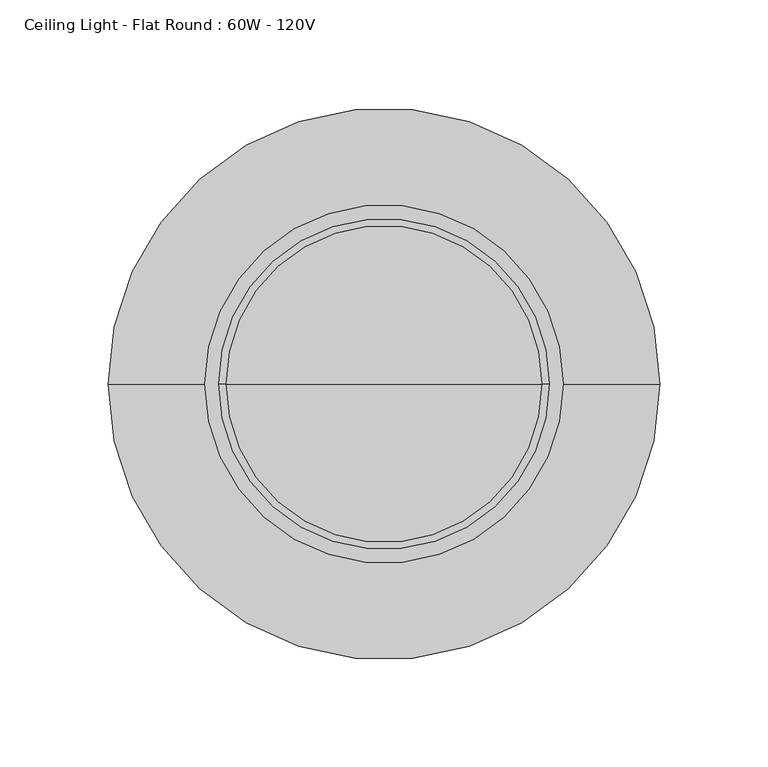
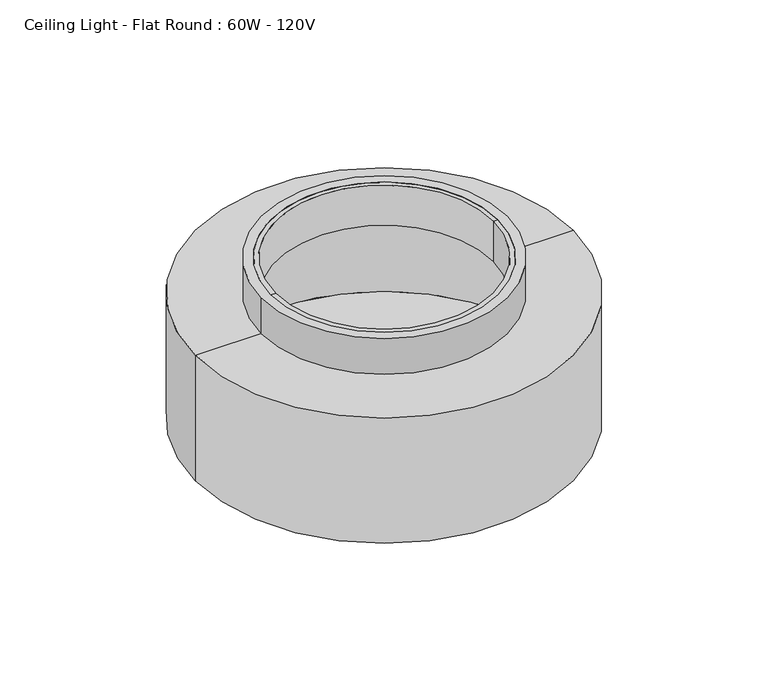
"""IFC4 building model written with IfcOpenShell, lengths in millimetres: light fixture geometry, Ceiling Light - Flat Round : 60W - 120V."""

from ifc_helpers import new_model, si_unit, point, frame, origin, origin_2d, place, context, project, spatial, polyline, circle_curve, trimmed, segment, composite_curve, outline, extrude, source, transform, mapped, element, save
from ifc_brep_helpers import plane_surface, cylinder_surface, revolved_surface, advanced_brep


def ceiling_light_flat_round_60w_120v_0a96185f(model_context):
    return source(origin(), model_context, "Body", "SolidModel", [
        extrude(outline(composite_curve([segment(trimmed(circle_curve(origin_2d(), 82.55), [point((-82.55, 0.0))], [point((82.55, 0.0))], False, "CARTESIAN"), True, "CONTINUOUS"), segment(trimmed(circle_curve(origin_2d(), 82.55), [point((82.55, 0.0))], [point((-82.55, 0.0))], False, "CARTESIAN"), True, "CONTINUOUS")], self_intersect=False), holes=[composite_curve([segment(trimmed(circle_curve(origin_2d(), 76.2), [point((-76.2, 0.0))], [point((76.2, 0.0))], True, "CARTESIAN"), True, "CONTINUOUS"), segment(trimmed(circle_curve(origin_2d(), 76.2), [point((76.2, 0.0))], [point((-76.2, 0.0))], True, "CARTESIAN"), True, "CONTINUOUS")], self_intersect=False)]), frame((0.0, 0.0, 2413.0), z_axis=(0.0, 0.0, 1.0), x_axis=(1.0, 0.0, 0.0)), (0.0, 0.0, 1.0), 25.4),
        advanced_brep(
        [(127.0, 0.0, 2413.0), (-127.0, 0.0, 2413.0), (-76.2, 0.0, 2413.0), (76.2, 0.0, 2413.0), (127.0, 0.0, 2324.1), (-127.0, 0.0, 2324.1), (0.0, 0.0, 2324.1), (123.825, 0.0, 2327.275), (-123.825, 0.0, 2327.275), (0.0, 0.0, 2327.275), (123.825, 0.0, 2409.825), (-123.825, 0.0, 2409.825), (73.025, 0.0, 2409.825), (-73.025, 0.0, 2409.825), (73.025, 0.0, 2438.4), (-73.025, 0.0, 2438.4), (76.2, 0.0, 2438.4), (-76.2, 0.0, 2438.4)],
        [
            (0, 1, circle_curve(frame((0.0, 0.0, 2413.0), z_axis=(0.0, 0.0, 1.0), x_axis=(-1.0, 0.0, 0.0)), 127.0)),
            (1, 2),
            (2, 3, circle_curve(frame((0.0, 0.0, 2413.0), z_axis=(0.0, 0.0, -1.0), x_axis=(-1.0, 0.0, 0.0)), 76.2)),
            (3, 0),
            (1, 0, circle_curve(frame((0.0, 0.0, 2413.0), z_axis=(0.0, 0.0, 1.0), x_axis=(-1.0, 0.0, 0.0)), 127.0)),
            (3, 2, circle_curve(frame((0.0, 0.0, 2413.0), z_axis=(0.0, 0.0, -1.0), x_axis=(-1.0, 0.0, 0.0)), 76.2)),
            (4, 5, circle_curve(frame((0.0, 0.0, 2324.1), z_axis=(0.0, 0.0, 1.0), x_axis=(-1.0, 0.0, 0.0)), 127.0)),
            (5, 1),
            (0, 4),
            (5, 4, circle_curve(frame((0.0, 0.0, 2324.1), z_axis=(0.0, 0.0, 1.0), x_axis=(-1.0, 0.0, 0.0)), 127.0)),
            (6, 5),
            (4, 6),
            (7, 8, circle_curve(frame((0.0, 0.0, 2327.275), z_axis=(0.0, 0.0, 1.0), x_axis=(-1.0, 0.0, 0.0)), 123.825)),
            (8, 9),
            (9, 7),
            (8, 7, circle_curve(frame((0.0, 0.0, 2327.275), z_axis=(0.0, 0.0, 1.0), x_axis=(-1.0, 0.0, 0.0)), 123.825)),
            (10, 11, circle_curve(frame((0.0, 0.0, 2409.825), z_axis=(0.0, 0.0, 1.0), x_axis=(-1.0, 0.0, 0.0)), 123.825)),
            (11, 8),
            (7, 10),
            (11, 10, circle_curve(frame((0.0, 0.0, 2409.825), z_axis=(0.0, 0.0, 1.0), x_axis=(-1.0, 0.0, 0.0)), 123.825)),
            (12, 13, circle_curve(frame((0.0, 0.0, 2409.825), z_axis=(0.0, 0.0, 1.0), x_axis=(-1.0, 0.0, 0.0)), 73.025)),
            (13, 11),
            (10, 12),
            (13, 12, circle_curve(frame((0.0, 0.0, 2409.825), z_axis=(0.0, 0.0, 1.0), x_axis=(-1.0, 0.0, 0.0)), 73.025)),
            (14, 15, circle_curve(frame((0.0, 0.0, 2438.4), z_axis=(0.0, 0.0, 1.0), x_axis=(-1.0, 0.0, 0.0)), 73.025)),
            (15, 13),
            (12, 14),
            (15, 14, circle_curve(frame((0.0, 0.0, 2438.4), z_axis=(0.0, 0.0, 1.0), x_axis=(-1.0, 0.0, 0.0)), 73.025)),
            (16, 17, circle_curve(frame((0.0, 0.0, 2438.4), z_axis=(0.0, 0.0, 1.0), x_axis=(-1.0, 0.0, 0.0)), 76.2)),
            (17, 15),
            (14, 16),
            (17, 16, circle_curve(frame((0.0, 0.0, 2438.4), z_axis=(0.0, 0.0, 1.0), x_axis=(-1.0, 0.0, 0.0)), 76.2)),
            (2, 17),
            (16, 3),
        ],
        [
            plane_surface(frame((0.0, 0.0, 2413.0), z_axis=(0.0, 0.0, 1.0), x_axis=(-1.0, 0.0, 0.0))),
            cylinder_surface(frame((0.0, 0.0, 2463.8), z_axis=(0.0, 0.0, -1.0), x_axis=(-1.0, 0.0, 0.0)), 127.0),
            plane_surface(frame((0.0, 0.0, 2324.1), z_axis=(0.0, 0.0, -1.0), x_axis=(-1.0, 0.0, 0.0))),
            plane_surface(frame((0.0, 0.0, 2327.275), z_axis=(0.0, 0.0, 1.0), x_axis=(-1.0, 0.0, 0.0))),
            revolved_surface(polyline([(-123.825, 0.0, 2327.275), (-123.825, 0.0, 2409.825)]), (0.0, 0.0, 2463.8), (0.0, 0.0, -1.0)),
            plane_surface(frame((0.0, 0.0, 2409.825), z_axis=(0.0, 0.0, -1.0), x_axis=(-1.0, 0.0, 0.0))),
            revolved_surface(polyline([(-73.025, 0.0, 2409.825), (-73.025, 0.0, 2438.4)]), (0.0, 0.0, 2463.8), (0.0, 0.0, -1.0)),
            plane_surface(frame((0.0, 0.0, 2438.4), z_axis=(0.0, 0.0, 1.0), x_axis=(-1.0, 0.0, 0.0))),
            cylinder_surface(frame((0.0, 0.0, 2463.8), z_axis=(0.0, 0.0, -1.0), x_axis=(-1.0, 0.0, 0.0)), 76.2),
        ],
        [
            (0, [[1, 2, 3, 4]]),
            (0, [[5, -4, 6, -2]]),
            (1, [[7, 8, -1, 9]]),
            (1, [[10, -9, -5, -8]]),
            (2, [[11, -7, 12]]),
            (2, [[-12, -10, -11]]),
            (3, [[13, 14, 15]]),
            (3, [[16, -15, -14]]),
            (4, [[17, 18, -13, 19]]),
            (4, [[20, -19, -16, -18]]),
            (5, [[21, 22, -17, 23]]),
            (5, [[24, -23, -20, -22]]),
            (6, [[25, 26, -21, 27]]),
            (6, [[28, -27, -24, -26]]),
            (7, [[29, 30, -25, 31]]),
            (7, [[32, -31, -28, -30]]),
            (8, [[-3, 33, -29, 34]]),
            (8, [[-6, -34, -32, -33]]),
        ],
    ),
    ])


if __name__ == "__main__":
    model = new_model("IFC4")
    model_context = context("Model", 3, world=origin())
    ifc_project = project(units=[si_unit("LENGTHUNIT", "METRE", prefix="MILLI")], contexts=[model_context])
    site = spatial("IfcSite", under=ifc_project)
    building = spatial("IfcBuilding", under=site)
    placement = place(None, origin())
    ceiling_light_flat_round_60w_120v_shape = ceiling_light_flat_round_60w_120v_0a96185f(model_context)
    element("IfcLightFixture", 1, ObjectType="Ceiling Light - Flat Round : 60W - 120V", at=placement, inside=building, context=model_context, shape_type="MappedRepresentation", body=[
        mapped(ceiling_light_flat_round_60w_120v_shape, transform((0.0, 0.0, 0.0), x_axis=(1.0, 0.0, 0.0), y_axis=(0.0, 1.0, 0.0), z_axis=(0.0, 0.0, 1.0))),
    ])
    save(model, "model.ifc")

# Revit data of these elements
# Type "Ceiling Light - Flat Round : 60W - 120V"
#   Lamp = "A-19"
#   Assembly Code = "D5020220"
#   Wattage = 60 W
#   built-in parameter 1150110 = 1 (stored number, unit not read)
#   built-in parameter 1114217 = 1 (stored number, unit not read)
#   built-in parameter 1150109 = 1 (stored number, unit not read)
#   built-in parameter 1150113 = 1 (stored number, unit not read)
#   built-in parameter 1150115 = 1 (stored number, unit not read)
#   built-in parameter 1150105 = 272.155 (stored number, unit not read)
#   Light Source Symbol Size = 2' - 0"
#   built-in parameter 1150112 = 1 (stored number, unit not read)
#   built-in parameter 1150114 = 1 (stored number, unit not read)
#   built-in parameter 1150107 = 2800 (stored number, unit not read)
#   built-in parameter 1150106 = 2.72155 (stored number, unit not read)
#   Emit from Circle Diameter = 0' - 10"
#   built-in parameter 1150104 = 1.32387 (stored number, unit not read)
#   Ballast Voltage = 120 V
#   built-in parameter 1114218 = 1 (stored number, unit not read)
#   built-in parameter 1150133 = 10 (stored number, unit not read)
#   Lumens = 855 lm
#   Apparent Load = 60 VA
#   built-in parameter 1150134 = 4
#   built-in parameter 1150137 = 1
#   Color Filter = 16777215
#   built-in parameter 1140040 [instance default] = 1
#   Ballast Number of Poles = 1
#   Light Box Material = Steel, Paint Finish, Dark Gray, Matte
#   Diffuser Material = Glass, White, High Luminance
#   Wattage Comments = ""
#   Emit Shape Visible in Rendering = no
#   Dimming Lamp Color Temperature Shift = (empty or 0)
#   Default Elevation = 0
# Element 1 (IfcLightFixture, "Ceiling Light - Flat Round : 60W - 120V")
#   Materials on its faces: "Glass, White, High Luminance", "Steel, Paint Finish, Dark Gray, Matte"
# Materials
#   "Steel, Paint Finish, Dark Gray, Matte": class "Metal", colour RGB 98 98 98, transparency 0, Description = "Steel, paint finish, dark gray, matte", Cost = 0
#   "Glass, White, High Luminance": class "Glass", colour RGB 249 250 249, transparency 0.8, Description = "physical material", Cost = 0
